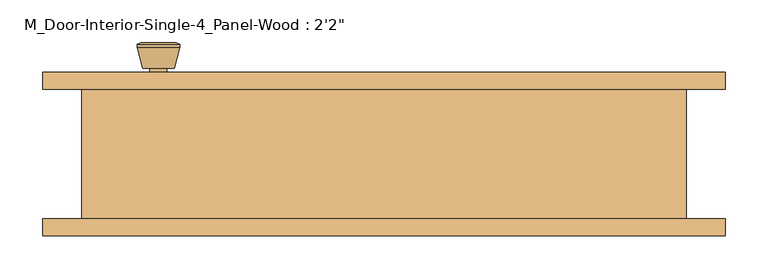
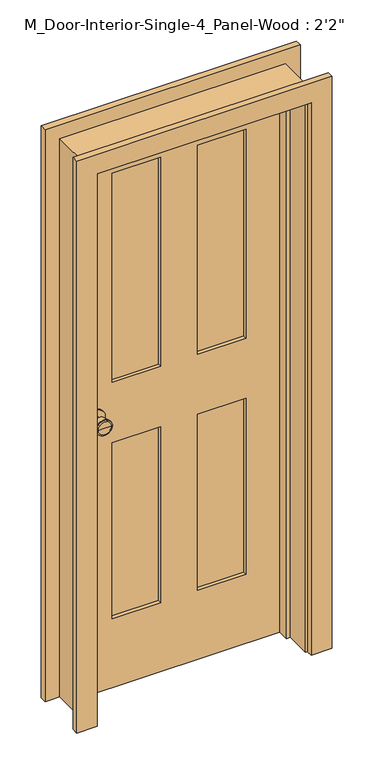
"""IFC4 building model written with IfcOpenShell, lengths in millimetres: door geometry."""

from ifc_helpers import new_model, si_unit, point, frame, frame_2d, origin, place, context, project, spatial, polyline, circle_curve, trimmed, segment, composite_curve, outline, extrude, faceted_brep, source, transform, mapped, element, save
from ifc_brep_helpers import plane_surface, cylinder_surface, revolved_surface, advanced_brep


def door_a03dd1d4(model_context):
    return source(origin(), model_context, "Body", "SolidModel", [
        advanced_brep(
        [(-265.2, 32.025, 914.4), (-255.2, 32.025, 914.4), (-275.2, 32.025, 914.4), (-244.7241324, -16.975, 914.4), (-265.2, -16.975, 914.4), (-285.6758676, -16.975, 914.4), (-240.2, -15.1471319, 914.4), (-290.2, -15.1471319, 914.4), (-240.2, -11.6834537, 914.4), (-290.2, -11.6834537, 914.4), (-246.563764, 13.025, 914.4), (-283.836236, 13.025, 914.4), (-255.2, 13.025, 914.4), (-275.2, 13.025, 914.4)],
        [
            (0, 1),
            (1, 2, circle_curve(frame((-265.2, 32.025, 914.4), z_axis=(0.0, 1.0, 0.0), x_axis=(-1.0, 0.0, 0.0)), 10.0)),
            (2, 0),
            (2, 1, circle_curve(frame((-265.2, 32.025, 914.4), z_axis=(0.0, 1.0, 0.0), x_axis=(-1.0, 0.0, 0.0)), 10.0)),
            (3, 4),
            (4, 5),
            (5, 3, circle_curve(frame((-265.2, -16.975, 914.4), z_axis=(0.0, -1.0, 0.0), x_axis=(-1.0, 0.0, 0.0)), 20.4758676)),
            (3, 5, circle_curve(frame((-265.2, -16.975, 914.4), z_axis=(0.0, -1.0, 0.0), x_axis=(-1.0, 0.0, 0.0)), 20.4758676)),
            (6, 3),
            (5, 7),
            (7, 6, circle_curve(frame((-265.2, -15.1471319, 914.4), z_axis=(0.0, -1.0, 0.0), x_axis=(-1.0, 0.0, 0.0)), 25.0)),
            (6, 7, circle_curve(frame((-265.2, -15.1471319, 914.4), z_axis=(0.0, -1.0, 0.0), x_axis=(-1.0, 0.0, 0.0)), 25.0)),
            (8, 6),
            (7, 9),
            (9, 8, circle_curve(frame((-265.2, -11.6834537, 914.4), z_axis=(0.0, -1.0, 0.0), x_axis=(-1.0, 0.0, 0.0)), 25.0)),
            (8, 9, circle_curve(frame((-265.2, -11.6834537, 914.4), z_axis=(0.0, -1.0, 0.0), x_axis=(-1.0, 0.0, 0.0)), 25.0)),
            (10, 8),
            (9, 11),
            (11, 10, circle_curve(frame((-265.2, 13.025, 914.4), z_axis=(0.0, -1.0, 0.0), x_axis=(-1.0, 0.0, 0.0)), 18.636236)),
            (10, 11, circle_curve(frame((-265.2, 13.025, 914.4), z_axis=(0.0, -1.0, 0.0), x_axis=(-1.0, 0.0, 0.0)), 18.636236)),
            (12, 10),
            (11, 13),
            (13, 12, circle_curve(frame((-265.2, 13.025, 914.4), z_axis=(0.0, -1.0, 0.0), x_axis=(-1.0, 0.0, 0.0)), 10.0)),
            (12, 13, circle_curve(frame((-265.2, 13.025, 914.4), z_axis=(0.0, -1.0, 0.0), x_axis=(-1.0, 0.0, 0.0)), 10.0)),
            (1, 12),
            (13, 2),
        ],
        [
            plane_surface(frame((-265.2, 32.025, 914.4), z_axis=(0.0, 1.0, 0.0), x_axis=(-1.0, 0.0, 0.0))),
            plane_surface(frame((-265.2, -16.975, 914.4), z_axis=(0.0, -1.0, 0.0), x_axis=(-1.0, 0.0, 0.0))),
            revolved_surface(polyline([(-285.6758676, -16.975, 914.4), (-290.2, -15.1471319, 914.4)]), (-265.2, 32.025, 914.4), (0.0, 1.0, 0.0)),
            cylinder_surface(frame((-265.2, 32.025, 914.4), z_axis=(0.0, 1.0, 0.0), x_axis=(-1.0, 0.0, 0.0)), 25.0),
            revolved_surface(polyline([(-290.2, -11.6834537, 914.4), (-283.836236, 13.025, 914.4)]), (-265.2, 32.025, 914.4), (0.0, 1.0, 0.0)),
            plane_surface(frame((-265.2, 13.025, 914.4), z_axis=(0.0, 1.0, 0.0), x_axis=(-1.0, 0.0, 0.0))),
            cylinder_surface(frame((-265.2, 32.025, 914.4), z_axis=(0.0, 1.0, 0.0), x_axis=(-1.0, 0.0, 0.0)), 10.0),
        ],
        [
            (0, [[1, 2, 3]]),
            (0, [[-3, 4, -1]]),
            (1, [[5, 6, 7]]),
            (1, [[-6, -5, 8]]),
            (2, [[9, -7, 10, 11]]),
            (2, [[-10, -8, -9, 12]]),
            (3, [[13, -11, 14, 15]]),
            (3, [[-14, -12, -13, 16]]),
            (4, [[17, -15, 18, 19]]),
            (4, [[-18, -16, -17, 20]]),
            (5, [[21, -19, 22, 23]]),
            (5, [[-22, -20, -21, 24]]),
            (6, [[25, -23, 26, -2]]),
            (6, [[-26, -24, -25, -4]]),
        ],
    ),
        extrude(outline(composite_curve([segment(trimmed(circle_curve(frame_2d((914.4, -265.2)), 30.0), [point((914.4, -295.2))], [point((914.4, -235.2))], False, "CARTESIAN"), True, "CONTINUOUS"), segment(trimmed(circle_curve(frame_2d((914.4, -265.2)), 30.0), [point((914.4, -235.2))], [point((914.4, -295.2))], False, "CARTESIAN"), True, "CONTINUOUS")], self_intersect=False)), frame((0.0, 32.025, 0.0), z_axis=(0.0, 1.0, 0.0), x_axis=(0.0, 0.0, 1.0)), (0.0, 0.0, 1.0), 6.0),
        advanced_brep(
        [(-265.2, 79.025, 914.4), (-275.2, 79.025, 914.4), (-255.2, 79.025, 914.4), (-244.7241324, 128.025, 914.4), (-285.6758676, 128.025, 914.4), (-265.2, 128.025, 914.4), (-240.2, 126.1971319, 914.4), (-290.2, 126.1971319, 914.4), (-240.2, 122.7334537, 914.4), (-290.2, 122.7334537, 914.4), (-246.563764, 98.025, 914.4), (-283.836236, 98.025, 914.4), (-255.2, 98.025, 914.4), (-275.2, 98.025, 914.4)],
        [
            (0, 1),
            (1, 2, circle_curve(frame((-265.2, 79.025, 914.4), z_axis=(0.0, -1.0, 0.0), x_axis=(-1.0, 0.0, 0.0)), 10.0)),
            (2, 0),
            (2, 1, circle_curve(frame((-265.2, 79.025, 914.4), z_axis=(0.0, -1.0, 0.0), x_axis=(-1.0, 0.0, 0.0)), 10.0)),
            (3, 4, circle_curve(frame((-265.2, 128.025, 914.4), z_axis=(0.0, 1.0, 0.0), x_axis=(-1.0, 0.0, 0.0)), 20.4758676)),
            (4, 5),
            (5, 3),
            (4, 3, circle_curve(frame((-265.2, 128.025, 914.4), z_axis=(0.0, 1.0, 0.0), x_axis=(-1.0, 0.0, 0.0)), 20.4758676)),
            (6, 7, circle_curve(frame((-265.2, 126.1971319, 914.4), z_axis=(0.0, 1.0, 0.0), x_axis=(-1.0, 0.0, 0.0)), 25.0)),
            (7, 4),
            (3, 6),
            (7, 6, circle_curve(frame((-265.2, 126.1971319, 914.4), z_axis=(0.0, 1.0, 0.0), x_axis=(-1.0, 0.0, 0.0)), 25.0)),
            (8, 9, circle_curve(frame((-265.2, 122.7334537, 914.4), z_axis=(0.0, 1.0, 0.0), x_axis=(-1.0, 0.0, 0.0)), 25.0)),
            (9, 7),
            (6, 8),
            (9, 8, circle_curve(frame((-265.2, 122.7334537, 914.4), z_axis=(0.0, 1.0, 0.0), x_axis=(-1.0, 0.0, 0.0)), 25.0)),
            (10, 11, circle_curve(frame((-265.2, 98.025, 914.4), z_axis=(0.0, 1.0, 0.0), x_axis=(-1.0, 0.0, 0.0)), 18.636236)),
            (11, 9),
            (8, 10),
            (11, 10, circle_curve(frame((-265.2, 98.025, 914.4), z_axis=(0.0, 1.0, 0.0), x_axis=(-1.0, 0.0, 0.0)), 18.636236)),
            (12, 13, circle_curve(frame((-265.2, 98.025, 914.4), z_axis=(0.0, 1.0, 0.0), x_axis=(-1.0, 0.0, 0.0)), 10.0)),
            (13, 11),
            (10, 12),
            (13, 12, circle_curve(frame((-265.2, 98.025, 914.4), z_axis=(0.0, 1.0, 0.0), x_axis=(-1.0, 0.0, 0.0)), 10.0)),
            (1, 13),
            (12, 2),
        ],
        [
            plane_surface(frame((-265.2, 79.025, 914.4), z_axis=(0.0, -1.0, 0.0), x_axis=(-1.0, 0.0, 0.0))),
            plane_surface(frame((-265.2, 128.025, 914.4), z_axis=(0.0, 1.0, 0.0), x_axis=(-1.0, 0.0, 0.0))),
            revolved_surface(polyline([(-285.6758676, 128.025, 914.4), (-290.2, 126.1971319, 914.4)]), (-265.2, 79.025, 914.4), (0.0, -1.0, 0.0)),
            cylinder_surface(frame((-265.2, 79.025, 914.4), z_axis=(0.0, -1.0, 0.0), x_axis=(-1.0, 0.0, 0.0)), 25.0),
            revolved_surface(polyline([(-290.2, 122.7334537, 914.4), (-283.836236, 98.025, 914.4)]), (-265.2, 79.025, 914.4), (0.0, -1.0, 0.0)),
            plane_surface(frame((-265.2, 98.025, 914.4), z_axis=(0.0, -1.0, 0.0), x_axis=(-1.0, 0.0, 0.0))),
            cylinder_surface(frame((-265.2, 79.025, 914.4), z_axis=(0.0, -1.0, 0.0), x_axis=(-1.0, 0.0, 0.0)), 10.0),
        ],
        [
            (0, [[1, 2, 3]]),
            (0, [[-3, 4, -1]]),
            (1, [[5, 6, 7]]),
            (1, [[8, -7, -6]]),
            (2, [[9, 10, -5, 11]]),
            (2, [[12, -11, -8, -10]]),
            (3, [[13, 14, -9, 15]]),
            (3, [[16, -15, -12, -14]]),
            (4, [[17, 18, -13, 19]]),
            (4, [[20, -19, -16, -18]]),
            (5, [[21, 22, -17, 23]]),
            (5, [[24, -23, -20, -22]]),
            (6, [[-2, 25, -21, 26]]),
            (6, [[-4, -26, -24, -25]]),
        ],
    ),
        extrude(outline(composite_curve([segment(trimmed(circle_curve(frame_2d((914.4, -265.2)), 30.0), [point((914.4, -295.2))], [point((914.4, -235.2))], False, "CARTESIAN"), True, "CONTINUOUS"), segment(trimmed(circle_curve(frame_2d((914.4, -265.2)), 30.0), [point((914.4, -235.2))], [point((914.4, -295.2))], False, "CARTESIAN"), True, "CONTINUOUS")], self_intersect=False)), frame((0.0, 73.025, 0.0), z_axis=(0.0, 1.0, 0.0), x_axis=(0.0, 0.0, 1.0)), (0.0, 0.0, 1.0), 6.0),
        faceted_brep([(355.2, 73.025, 0.0), (355.2, -79.375, 0.0), (330.2, -79.375, 0.0), (330.2, 3.1, 0.0), (317.5, 3.1, 0.0), (317.5, 38.025, 0.0), (330.2, 38.025, 0.0), (330.2, 73.025, 0.0), (355.2, 73.025, 1853.8), (355.2, -79.375, 1853.8), (-355.2, -79.375, 1853.8), (-355.2, -79.375, 0.0), (-330.2, -79.375, 0.0), (-330.2, -79.375, 1828.8), (330.2, -79.375, 1828.8), (330.2, 3.1, 1828.8), (-330.2, 3.1, 1828.8), (-330.2, 3.1, 0.0), (-317.5, 3.1, 0.0), (-317.5, 3.1, 1816.1), (317.5, 3.1, 1816.1), (317.5, 38.025, 1816.1), (-317.5, 38.025, 1816.1), (-317.5, 38.025, 0.0), (-330.2, 38.025, 0.0), (-330.2, 38.025, 1828.8), (330.2, 38.025, 1828.8), (330.2, 73.025, 1828.8), (-330.2, 73.025, 1828.8), (-330.2, 73.025, 0.0), (-355.2, 73.025, 0.0), (-355.2, 73.025, 1853.8)], [[[0, 1, 2, 3, 4, 5, 6, 7]], [[1, 0, 8, 9]], [[2, 1, 9, 10, 11, 12, 13, 14]], [[3, 2, 14, 15]], [[4, 3, 15, 16, 17, 18, 19, 20]], [[5, 4, 20, 21]], [[6, 5, 21, 22, 23, 24, 25, 26]], [[7, 6, 26, 27]], [[0, 7, 27, 28, 29, 30, 31, 8]], [[9, 8, 31, 10]], [[15, 14, 13, 16]], [[21, 20, 19, 22]], [[27, 26, 25, 28]], [[30, 29, 24, 23, 18, 17, 12, 11]], [[10, 31, 30, 11]], [[16, 13, 12, 17]], [[22, 19, 18, 23]], [[28, 25, 24, 29]]]),
        extrude(outline(polyline([(1828.8, -330.2), (0.0, -330.2), (0.0, 330.2), (1828.8, 330.2), (1828.8, -330.2)]), holes=[polyline([(1708.8, 57.5), (1708.8, 210.2), (1014.4, 210.2), (1014.4, 57.5), (1708.8, 57.5)]), polyline([(1014.4, -57.5), (1014.4, -210.2), (1708.8, -210.2), (1708.8, -57.5), (1014.4, -57.5)]), polyline([(814.4, 57.5), (814.4, 210.2), (230.0, 210.2), (230.0, 57.5), (814.4, 57.5)]), polyline([(230.0, -57.5), (230.0, -210.2), (814.4, -210.2), (814.4, -57.5), (230.0, -57.5)])]), frame((0.0, 38.025, 0.0), z_axis=(0.0, 1.0, 0.0), x_axis=(0.0, 0.0, 1.0)), (0.0, 0.0, 1.0), 35.0),
        extrude(outline(polyline([(210.2, 49.6916667), (57.5, 49.6916667), (57.5, 61.3583333), (210.2, 61.3583333), (210.2, 49.6916667)])), frame((0.0, 0.0, 1014.4), z_axis=(0.0, 0.0, 1.0), x_axis=(1.0, 0.0, 0.0)), (0.0, 0.0, 1.0), 694.4),
        extrude(outline(polyline([(-57.5, 49.6916667), (-210.2, 49.6916667), (-210.2, 61.3583333), (-57.5, 61.3583333), (-57.5, 49.6916667)])), frame((0.0, 0.0, 1014.4), z_axis=(0.0, 0.0, 1.0), x_axis=(1.0, 0.0, 0.0)), (0.0, 0.0, 1.0), 694.4),
        extrude(outline(polyline([(210.2, 49.6916667), (57.5, 49.6916667), (57.5, 61.3583333), (210.2, 61.3583333), (210.2, 49.6916667)])), frame((0.0, 0.0, 230.0), z_axis=(0.0, 0.0, 1.0), x_axis=(1.0, 0.0, 0.0)), (0.0, 0.0, 1.0), 584.4),
        extrude(outline(polyline([(-57.5, 49.6916667), (-210.2, 49.6916667), (-210.2, 61.3583333), (-57.5, 61.3583333), (-57.5, 49.6916667)])), frame((0.0, 0.0, 230.0), z_axis=(0.0, 0.0, 1.0), x_axis=(1.0, 0.0, 0.0)), (0.0, 0.0, 1.0), 584.4),
        extrude(outline(polyline([(0.0, 336.55), (0.0, 401.55), (1900.15, 401.55), (1900.15, -401.55), (0.0, -401.55), (0.0, -336.55), (1835.15, -336.55), (1835.15, 336.55), (0.0, 336.55)])), frame((0.0, 73.025, 0.0), z_axis=(0.0, 1.0, 0.0), x_axis=(0.0, 0.0, 1.0)), (0.0, 0.0, 1.0), 20.0),
        extrude(outline(polyline([(0.0, 336.55), (0.0, 401.55), (1900.15, 401.55), (1900.15, -401.55), (0.0, -401.55), (0.0, -336.55), (1835.15, -336.55), (1835.15, 336.55), (0.0, 336.55)])), frame((0.0, -99.375, 0.0), z_axis=(0.0, 1.0, 0.0), x_axis=(0.0, 0.0, 1.0)), (0.0, 0.0, 1.0), 20.0),
    ])


if __name__ == "__main__":
    model = new_model("IFC4")
    model_context = context("Model", 3, world=origin())
    ifc_project = project(units=[si_unit("LENGTHUNIT", "METRE", prefix="MILLI")], contexts=[model_context])
    site = spatial("IfcSite", under=ifc_project)
    building = spatial("IfcBuilding", under=site)
    placement = place(None, origin())
    door_shape = door_a03dd1d4(model_context)
    element("IfcDoor", 1, ObjectType="M_Door-Interior-Single-4_Panel-Wood : 2'2\"", at=placement, inside=building, context=model_context, shape_type="MappedRepresentation", body=[
        mapped(door_shape, transform((0.0, 0.0, 0.0), x_axis=(1.0, 0.0, 0.0), y_axis=(0.0, 1.0, 0.0), z_axis=(0.0, 0.0, 1.0))),
    ])
    save(model, "model.ifc")

# Revit data of these elements
# Type "M_Door-Interior-Single-4_Panel-Wood : 2'2\""
#   Type Mark = "43"
#   Assembly Code = "C1020300"
#   Analytic Construction = "Wooden"
#   Top Rail = 0' - 4.72441"
#   Thickness = 0' - 1.37795"
#   Thermal Resistance (R) = 0.455703 (m²·K)/W
#   Swing Angle [instance default] = 90.00°
#   Stiles = 0' - 4.72441"
#   Rough Width = 2' - 3.9685"
#   Rough Height = 6' - 0.98425"
#   Mullion = 0' - 4.52756"
#   Lock Rail = 0' - 7.87402"
#   Height = 6' - 0"
#   Width = 2' - 2"
#   Heat Transfer Coefficient (U) = 2.19465 W/(m²·K)
#   Bottom Rail = 0' - 9.05512"
#   Trim Material = Cherry
#   Panel Material = Cherry
#   Frame Material = Cherry
#   Door Handle Material = Aluminum
#   Visual Light Transmittance = 0
#   Solar Heat Gain Coefficient = 0
#   Wall Closure = (empty or 0)
#   Function = (empty or 0)
# Element 1 (IfcDoor, "M_Door-Interior-Single-4_Panel-Wood : 2'2\"")
#   Materials on its faces: "Cherry", "Aluminum"
# Materials
#   "Cherry": class "Wood", colour RGB 226 177 128, transparency 0, Description = "Prunus Serotina", Cost = 0
#   "Aluminum": class "Metal", colour RGB 247 247 247, transparency 0, Description = "Aluminum 6061", Cost = 0
